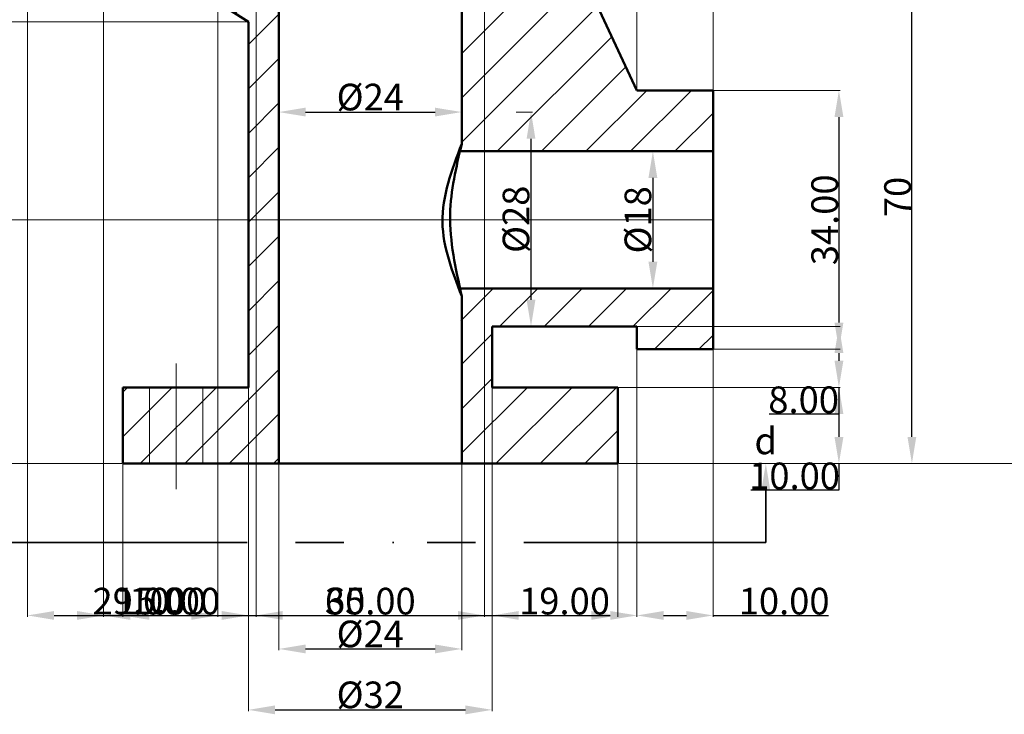
# Model space of a CAD drawing. Units: millimetres. Extents: x 75 to 489, y 21 to 350.
# Tile 3 of 5: x 142 to 271, y 176 to 268. Entities that reach past the tile are written whole.
import ezdxf

# ---------------------------------------------------------------- set-up
doc = ezdxf.new("R2010")
doc.units = ezdxf.units.MM
doc.header["$MEASUREMENT"] = 0
doc.linetypes.add('CENTER', pattern=[50.8, 31.75, -6.35, 6.35, -6.35])
doc.linetypes.add('PHANTOM', pattern=[63.5, 31.75, -6.35, 6.35, -6.35, 6.35, -6.35])
for name, color, linetype, lineweight in [('M-CNTR', 1, 'CENTER', 18), ('M-DIMS', 2, 'Continuous', 25), ('M-HATC', 8, 'Continuous', 18), ('M-OUTL', 7, 'Continuous', 50), ('M-SECT', 3, 'PHANTOM', 35), ('M-TEXT', 7, 'Continuous', 25), ('M-THRD', 3, 'Continuous', 18)]:
    doc.layers.add(name, color=color, linetype=linetype, lineweight=lineweight)
doc.styles.get("Standard").update_dxf_attribs({"font": 'arial.ttf'})
doc.dimstyles.get("Standard").update_dxf_attribs({"dimtxt": 3.5, "dimasz": 3.5, "dimexe": 0.18, "dimexo": 0.0625, "dimgap": 0.09, "dimtad": 1, "dimtoh": 1, "dimdec": 0, "dimzin": 0, "dimdsep": 46, "dimtxsty": 'Standard', "dimcen": 0.09, "dimclrd": 2, "dimclre": 251, "dimadec": 0, "dimazin": 0, "dimtfac": 1, "dimtdec": 0, "dimtofl": 0, "dimtmove": 0, "dimatfit": 3, "dimfxl": 1, "dimtolj": 1, "dimtzin": 0, "dimlwe": 5, "dimarcsym": 0})

# ---------------------------------------------------------------- blocks, each defined once
blk = doc.blocks.new('*D19')
at = {"layer": 'Defpoints', "color": 0, "transparency": 16777216}
for p in [(203.9, 223.35), (171.9, 219.35), (203.9, 177)]:
    blk.add_point(p, dxfattribs=at)
at = {"layer": 'M-DIMS', "color": 0, "lineweight": 5, "transparency": 16777216}
for p, q in [((203.9, 223.28), (203.9, 176.82)), ((171.9, 219.28), (171.9, 176.82))]:
    blk.add_line(p, q, dxfattribs=at)
at = {"layer": 'M-DIMS', "color": 0, "lineweight": -2, "transparency": 16777216}
blk.add_line((175.4, 177), (200.4, 177), dxfattribs=at)
at = {"layer": 'M-DIMS', "color": 0, "transparency": 16777216}
for points in [[(175.4, 177.58), (175.4, 176.42), (171.9, 177)], [(200.4, 177.58), (200.4, 176.42), (203.9, 177)]]:
    blk.add_solid(points, dxfattribs=at)
at = {"layer": 'M-DIMS', "color": 0, "transparency": 16777216, "insert": (187.9, 178.97), "char_height": 3.5, "attachment_point": 5}
blk.add_mtext('\\A1;%%C32', dxfattribs=at)
blk = doc.blocks.new('*D20')
at = {"layer": 'Defpoints', "color": 0, "transparency": 16777216}
for p in [(175.9, 216), (199.9, 216), (199.9, 185)]:
    blk.add_point(p, dxfattribs=at)
at = {"layer": 'M-DIMS', "color": 0, "lineweight": 5, "transparency": 16777216}
for p, q in [((175.9, 215.94), (175.9, 184.82)), ((199.9, 215.94), (199.9, 184.82))]:
    blk.add_line(p, q, dxfattribs=at)
at = {"layer": 'M-DIMS', "color": 0, "lineweight": -2, "transparency": 16777216}
blk.add_line((179.4, 185), (196.4, 185), dxfattribs=at)
at = {"layer": 'M-DIMS', "color": 0, "transparency": 16777216}
for points in [[(179.4, 185.58), (179.4, 184.42), (175.9, 185)], [(196.4, 185.58), (196.4, 184.42), (199.9, 185)]]:
    blk.add_solid(points, dxfattribs=at)
at = {"layer": 'M-DIMS', "color": 0, "transparency": 16777216, "insert": (187.9, 186.97), "char_height": 3.5, "attachment_point": 5}
blk.add_mtext('\\A1;%%C24', dxfattribs=at)
blk = doc.blocks.new('*D25')
at = {"layer": 'Defpoints', "color": 0, "transparency": 16777216}
for p in [(142.9, 299.35), (125.5, 241.35), (232.9, 241.35)]:
    blk.add_point(p, dxfattribs=at)
at = {"layer": 'M-DIMS', "color": 0, "lineweight": 5, "transparency": 16777216}
for p, q in [((142.84, 299.35), (125.32, 299.35)), ((232.84, 241.35), (125.32, 241.35))]:
    blk.add_line(p, q, dxfattribs=at)
at = {"layer": 'M-DIMS', "color": 0, "lineweight": -2, "transparency": 16777216}
blk.add_line((125.5, 295.85), (125.5, 244.85), dxfattribs=at)
at = {"layer": 'M-DIMS', "color": 0, "transparency": 16777216}
for points in [[(124.92, 295.85), (126.08, 295.85), (125.5, 299.35)], [(124.92, 244.85), (126.08, 244.85), (125.5, 241.35)]]:
    blk.add_solid(points, dxfattribs=at)
at = {"layer": 'M-DIMS', "color": 0, "transparency": 16777216, "insert": (123.62, 270.35), "char_height": 3.5, "attachment_point": 5, "rotation": 90}
blk.add_mtext('\\A1;58', dxfattribs=at)
blk = doc.blocks.new('*D26')
at = {"layer": 'Defpoints', "color": 0, "transparency": 16777216}
for p in [(117, 299.35), (142.9, 299.35), (155.4, 209.35)]:
    blk.add_point(p, dxfattribs=at)
at = {"layer": 'M-DIMS', "color": 0, "lineweight": 5, "transparency": 16777216}
for p, q in [((142.84, 299.35), (116.82, 299.35)), ((155.34, 209.35), (116.82, 209.35))]:
    blk.add_line(p, q, dxfattribs=at)
at = {"layer": 'M-DIMS', "color": 0, "lineweight": -2, "transparency": 16777216}
blk.add_line((117, 212.85), (117, 295.85), dxfattribs=at)
at = {"layer": 'M-DIMS', "color": 0, "transparency": 16777216}
for points in [[(116.42, 295.85), (117.58, 295.85), (117, 299.35)], [(116.42, 212.85), (117.58, 212.85), (117, 209.35)]]:
    blk.add_solid(points, dxfattribs=at)
at = {"layer": 'M-DIMS', "color": 0, "transparency": 16777216, "insert": (115.12, 254.35), "char_height": 3.5, "attachment_point": 5, "rotation": 90}
blk.add_mtext('\\A1;90', dxfattribs=at)
blk = doc.blocks.new('*D27')
at = {"layer": 'Defpoints', "color": 0, "transparency": 16777216}
for p in [(171.9, 267.35), (134, 209.35), (155.4, 209.35)]:
    blk.add_point(p, dxfattribs=at)
at = {"layer": 'M-DIMS', "color": 0, "lineweight": 5, "transparency": 16777216}
for p, q in [((171.84, 267.35), (133.82, 267.35)), ((155.34, 209.35), (133.82, 209.35))]:
    blk.add_line(p, q, dxfattribs=at)
at = {"layer": 'M-DIMS', "color": 0, "lineweight": -2, "transparency": 16777216}
blk.add_line((134, 263.85), (134, 212.85), dxfattribs=at)
at = {"layer": 'M-DIMS', "color": 0, "transparency": 16777216}
for points in [[(133.42, 263.85), (134.58, 263.85), (134, 267.35)], [(133.42, 212.85), (134.58, 212.85), (134, 209.35)]]:
    blk.add_solid(points, dxfattribs=at)
at = {"layer": 'M-DIMS', "color": 0, "transparency": 16777216, "insert": (132.12, 238.35), "char_height": 3.5, "attachment_point": 5, "rotation": 90}
blk.add_mtext('\\A1;58', dxfattribs=at)
blk = doc.blocks.new('*D28')
at = {"layer": 'Defpoints', "color": 0, "transparency": 16777216}
for p in [(175.9, 255.5), (199.9, 255.5), (199.9, 255.5)]:
    blk.add_point(p, dxfattribs=at)
at = {"layer": 'M-DIMS', "color": 0, "lineweight": 5, "transparency": 16777216}
for p, q in [((175.9, 255.56), (175.9, 255.68)), ((199.9, 255.56), (199.9, 255.68))]:
    blk.add_line(p, q, dxfattribs=at)
at = {"layer": 'M-DIMS', "color": 0, "lineweight": -2, "transparency": 16777216}
blk.add_line((179.4, 255.5), (196.4, 255.5), dxfattribs=at)
at = {"layer": 'M-DIMS', "color": 0, "transparency": 16777216}
for points in [[(179.4, 256.08), (179.4, 254.92), (175.9, 255.5)], [(196.4, 256.08), (196.4, 254.92), (199.9, 255.5)]]:
    blk.add_solid(points, dxfattribs=at)
at = {"layer": 'M-DIMS', "color": 0, "transparency": 16777216, "insert": (187.9, 257.47), "char_height": 3.5, "attachment_point": 5}
blk.add_mtext('\\A1;%%C24', dxfattribs=at)
blk = doc.blocks.new('*D29')
at = {"layer": 'Defpoints', "color": 0, "transparency": 16777216}
for p in [(228.5, 250.35), (225, 232.35), (228.5, 232.35)]:
    blk.add_point(p, dxfattribs=at)
at = {"layer": 'M-DIMS', "color": 0, "lineweight": 5, "transparency": 16777216}
for p, q in [((228.44, 250.35), (224.82, 250.35)), ((228.44, 232.35), (224.82, 232.35))]:
    blk.add_line(p, q, dxfattribs=at)
at = {"layer": 'M-DIMS', "color": 0, "lineweight": -2, "transparency": 16777216}
blk.add_line((225, 246.85), (225, 235.85), dxfattribs=at)
at = {"layer": 'M-DIMS', "color": 0, "transparency": 16777216}
for points in [[(224.42, 246.85), (225.58, 246.85), (225, 250.35)], [(224.42, 235.85), (225.58, 235.85), (225, 232.35)]]:
    blk.add_solid(points, dxfattribs=at)
at = {"layer": 'M-DIMS', "color": 0, "transparency": 16777216, "insert": (223.03, 241.35), "char_height": 3.5, "width": 5.2587, "attachment_point": 5, "rotation": 90}
blk.add_mtext('\\A1;%%C18', dxfattribs=at)
blk = doc.blocks.new('*D30')
at = {"layer": 'Defpoints', "color": 0, "transparency": 16777216}
for p in [(207, 255.5), (209, 255.5), (207, 227.35)]:
    blk.add_point(p, dxfattribs=at)
at = {"layer": 'M-DIMS', "color": 0, "lineweight": 5, "transparency": 16777216}
for p, q in [((207.06, 255.5), (209.18, 255.5)), ((207.06, 227.35), (209.18, 227.35))]:
    blk.add_line(p, q, dxfattribs=at)
at = {"layer": 'M-DIMS', "color": 0, "lineweight": -2, "transparency": 16777216}
blk.add_line((209, 230.85), (209, 252), dxfattribs=at)
at = {"layer": 'M-DIMS', "color": 0, "transparency": 16777216}
for points in [[(208.42, 252), (209.58, 252), (209, 255.5)], [(208.42, 230.85), (209.58, 230.85), (209, 227.35)]]:
    blk.add_solid(points, dxfattribs=at)
at = {"layer": 'M-DIMS', "color": 0, "transparency": 16777216, "insert": (207.03, 241.42), "char_height": 3.5, "attachment_point": 5, "rotation": 90}
blk.add_mtext('\\A1;%%C28', dxfattribs=at)
blk = doc.blocks.new('*D31')
at = {"layer": 'Defpoints', "color": 0, "transparency": 16777216}
for p in [(199.9, 279.35), (259, 279.35), (220.4, 209.35)]:
    blk.add_point(p, dxfattribs=at)
at = {"layer": 'M-DIMS', "color": 0, "lineweight": 5, "transparency": 16777216}
for p, q in [((199.97, 279.35), (259.18, 279.35)), ((220.47, 209.35), (259.18, 209.35))]:
    blk.add_line(p, q, dxfattribs=at)
at = {"layer": 'M-DIMS', "color": 0, "lineweight": -2, "transparency": 16777216}
blk.add_line((259, 212.85), (259, 275.85), dxfattribs=at)
at = {"layer": 'M-DIMS', "color": 0, "transparency": 16777216}
for points in [[(258.42, 275.85), (259.58, 275.85), (259, 279.35)], [(258.42, 212.85), (259.58, 212.85), (259, 209.35)]]:
    blk.add_solid(points, dxfattribs=at)
at = {"layer": 'M-DIMS', "color": 0, "transparency": 16777216, "insert": (257.12, 244.35), "char_height": 3.5, "attachment_point": 5, "rotation": 90}
blk.add_mtext('\\A1;70', dxfattribs=at)
blk = doc.blocks.new('*D35')
at = {"layer": 'Defpoints', "color": 0, "transparency": 16777216}
for p in [(220.88, 327.35), (259, 209.35), (279.5, 209.35)]:
    blk.add_point(p, dxfattribs=at)
at = {"layer": 'M-DIMS', "color": 0, "lineweight": 5, "transparency": 16777216}
for p, q in [((220.95, 327.35), (279.68, 327.35)), ((259.06, 209.35), (279.68, 209.35))]:
    blk.add_line(p, q, dxfattribs=at)
at = {"layer": 'M-DIMS', "color": 0, "lineweight": -2, "transparency": 16777216}
blk.add_line((279.5, 323.85), (279.5, 212.85), dxfattribs=at)
at = {"layer": 'M-DIMS', "color": 0, "transparency": 16777216}
for points in [[(278.92, 323.85), (280.08, 323.85), (279.5, 327.35)], [(278.92, 212.85), (280.08, 212.85), (279.5, 209.35)]]:
    blk.add_solid(points, dxfattribs=at)
at = {"layer": 'M-DIMS', "color": 0, "transparency": 16777216, "insert": (277.62, 268.35), "char_height": 3.5, "attachment_point": 5, "rotation": 90}
blk.add_mtext('\\A1;118', dxfattribs=at)
blk = doc.blocks.new('*D44')
at = {"layer": 'Defpoints', "color": 0, "transparency": 16777216}
for p in [(232.9, 345.6), (142.9, 319.35), (232.9, 258.35)]:
    blk.add_point(p, dxfattribs=at)
at = {"layer": 'M-DIMS', "color": 251, "lineweight": 5, "transparency": 16777216}
for p, q in [((142.9, 319.41), (142.9, 345.78)), ((232.9, 258.41), (232.9, 345.78))]:
    blk.add_line(p, q, dxfattribs=at)
at = {"layer": 'M-DIMS', "color": 2, "lineweight": -2, "transparency": 16777216}
blk.add_line((146.4, 345.6), (229.4, 345.6), dxfattribs=at)
at = {"layer": 'M-DIMS', "color": 2, "transparency": 16777216}
for points in [[(146.4, 346.18), (146.4, 345.02), (142.9, 345.6)], [(229.4, 346.18), (229.4, 345.02), (232.9, 345.6)]]:
    blk.add_solid(points, dxfattribs=at)
at = {"layer": 'M-DIMS', "color": 0, "transparency": 16777216, "insert": (187.9, 347.48), "char_height": 3.5, "attachment_point": 5}
blk.add_mtext('\\A1;90.00', dxfattribs=at)
blk = doc.blocks.new('*D47')
at = {"layer": 'Defpoints', "color": 0, "transparency": 16777216}
for p in [(155.4, 209.35), (220.4, 209.35), (220.4, 189.4)]:
    blk.add_point(p, dxfattribs=at)
at = {"layer": 'M-DIMS', "color": 251, "lineweight": 5, "transparency": 16777216}
for p, q in [((155.4, 209.28), (155.4, 189.22)), ((220.4, 209.28), (220.4, 189.22))]:
    blk.add_line(p, q, dxfattribs=at)
at = {"layer": 'M-DIMS', "color": 2, "lineweight": -2, "transparency": 16777216}
blk.add_line((158.9, 189.4), (216.9, 189.4), dxfattribs=at)
at = {"layer": 'M-DIMS', "color": 2, "transparency": 16777216}
for points in [[(158.9, 189.98), (158.9, 188.82), (155.4, 189.4)], [(216.9, 189.98), (216.9, 188.82), (220.4, 189.4)]]:
    blk.add_solid(points, dxfattribs=at)
at = {"layer": 'M-DIMS', "color": 0, "transparency": 16777216, "insert": (187.9, 191.28), "char_height": 3.5, "attachment_point": 5}
blk.add_mtext('\\A1;65.00', dxfattribs=at)
blk = doc.blocks.new('*D48')
at = {"layer": 'Defpoints', "color": 0, "transparency": 16777216}
for p in [(220.4, 219.35), (220.4, 209.35), (249.42, 209.35)]:
    blk.add_point(p, dxfattribs=at)
at = {"layer": 'M-DIMS', "color": 251, "lineweight": 5, "transparency": 16777216}
for p, q in [((220.47, 219.35), (249.6, 219.35)), ((220.47, 209.35), (249.6, 209.35))]:
    blk.add_line(p, q, dxfattribs=at)
at = {"layer": 'M-DIMS', "color": 2, "lineweight": -2, "transparency": 16777216}
for p, q in [((249.42, 215.85), (249.42, 212.85)), ((249.42, 209.35), (249.42, 205.85)), ((249.42, 205.85), (237.86, 205.85))]:
    blk.add_line(p, q, dxfattribs=at)
at = {"layer": 'M-DIMS', "color": 2, "transparency": 16777216}
for points in [[(248.84, 215.85), (250.01, 215.85), (249.42, 219.35)], [(248.84, 212.85), (250.01, 212.85), (249.42, 209.35)]]:
    blk.add_solid(points, dxfattribs=at)
at = {"layer": 'M-DIMS', "color": 0, "transparency": 16777216, "insert": (243.6, 207.72), "char_height": 3.5, "attachment_point": 5}
blk.add_mtext('\\A1;10.00', dxfattribs=at)
blk = doc.blocks.new('*D50')
at = {"layer": 'Defpoints', "color": 0, "transparency": 16777216}
for p in [(142.9, 279.35), (152.9, 279.35), (152.9, 189.4)]:
    blk.add_point(p, dxfattribs=at)
at = {"layer": 'M-DIMS', "color": 251, "lineweight": 5, "transparency": 16777216}
for p, q in [((142.9, 279.28), (142.9, 189.22)), ((152.9, 279.28), (152.9, 189.22))]:
    blk.add_line(p, q, dxfattribs=at)
at = {"layer": 'M-DIMS', "color": 2, "lineweight": -2, "transparency": 16777216}
for p, q in [((146.4, 189.4), (149.4, 189.4)), ((152.9, 189.4), (168.05, 189.4))]:
    blk.add_line(p, q, dxfattribs=at)
at = {"layer": 'M-DIMS', "color": 2, "transparency": 16777216}
for points in [[(146.4, 189.98), (146.4, 188.82), (142.9, 189.4)], [(149.4, 189.98), (149.4, 188.82), (152.9, 189.4)]]:
    blk.add_solid(points, dxfattribs=at)
at = {"layer": 'M-DIMS', "color": 0, "transparency": 16777216, "insert": (162.23, 191.28), "char_height": 3.5, "attachment_point": 5}
blk.add_mtext('\\A1;10.00', dxfattribs=at)
blk = doc.blocks.new('*D51')
at = {"layer": 'Defpoints', "color": 0, "transparency": 16777216}
for p in [(142.9, 279.35), (171.9, 267.35), (171.9, 189.4)]:
    blk.add_point(p, dxfattribs=at)
at = {"layer": 'M-DIMS', "color": 251, "lineweight": 5, "transparency": 16777216}
for p, q in [((142.9, 279.28), (142.9, 189.22)), ((171.9, 267.28), (171.9, 189.22))]:
    blk.add_line(p, q, dxfattribs=at)
at = {"layer": 'M-DIMS', "color": 2, "lineweight": -2, "transparency": 16777216}
blk.add_line((146.4, 189.4), (168.4, 189.4), dxfattribs=at)
at = {"layer": 'M-DIMS', "color": 2, "transparency": 16777216}
for points in [[(146.4, 189.98), (146.4, 188.82), (142.9, 189.4)], [(168.4, 189.98), (168.4, 188.82), (171.9, 189.4)]]:
    blk.add_solid(points, dxfattribs=at)
at = {"layer": 'M-DIMS', "color": 0, "transparency": 16777216, "insert": (157.4, 191.28), "char_height": 3.5, "attachment_point": 5}
blk.add_mtext('\\A1;29.00', dxfattribs=at)
blk = doc.blocks.new('*D52')
at = {"layer": 'Defpoints', "color": 0, "transparency": 16777216}
for p in [(222.9, 345.6), (207.9, 290.35), (222.9, 258.35)]:
    blk.add_point(p, dxfattribs=at)
at = {"layer": 'M-DIMS', "color": 251, "lineweight": 5, "transparency": 16777216}
for p, q in [((207.9, 290.41), (207.9, 345.78)), ((222.9, 258.41), (222.9, 345.78))]:
    blk.add_line(p, q, dxfattribs=at)
at = {"layer": 'M-DIMS', "color": 2, "lineweight": -2, "transparency": 16777216}
blk.add_line((211.4, 345.6), (219.4, 345.6), dxfattribs=at)
at = {"layer": 'M-DIMS', "color": 2, "transparency": 16777216}
for points in [[(211.4, 346.18), (211.4, 345.02), (207.9, 345.6)], [(219.4, 346.18), (219.4, 345.02), (222.9, 345.6)]]:
    blk.add_solid(points, dxfattribs=at)
at = {"layer": 'M-DIMS', "color": 0, "transparency": 16777216, "insert": (215.4, 347.48), "char_height": 3.5, "attachment_point": 5}
blk.add_mtext('\\A1;15.00', dxfattribs=at)
blk = doc.blocks.new('*D53')
at = {"layer": 'Defpoints', "color": 0, "transparency": 16777216}
for p in [(152.9, 315.35), (167.9, 315.35), (167.9, 189.4)]:
    blk.add_point(p, dxfattribs=at)
at = {"layer": 'M-DIMS', "color": 251, "lineweight": 5, "transparency": 16777216}
for p, q in [((152.9, 315.28), (152.9, 189.22)), ((167.9, 315.28), (167.9, 189.22))]:
    blk.add_line(p, q, dxfattribs=at)
at = {"layer": 'M-DIMS', "color": 2, "lineweight": -2, "transparency": 16777216}
blk.add_line((156.4, 189.4), (164.4, 189.4), dxfattribs=at)
at = {"layer": 'M-DIMS', "color": 2, "transparency": 16777216}
for points in [[(156.4, 189.98), (156.4, 188.82), (152.9, 189.4)], [(164.4, 189.98), (164.4, 188.82), (167.9, 189.4)]]:
    blk.add_solid(points, dxfattribs=at)
at = {"layer": 'M-DIMS', "color": 0, "transparency": 16777216, "insert": (160.4, 191.28), "char_height": 3.5, "attachment_point": 5}
blk.add_mtext('\\A1;15.00', dxfattribs=at)
blk = doc.blocks.new('*D54')
at = {"layer": 'Defpoints', "color": 0, "transparency": 16777216}
for p in [(232.9, 258.35), (232.9, 224.35), (249.42, 224.35)]:
    blk.add_point(p, dxfattribs=at)
at = {"layer": 'M-DIMS', "color": 251, "lineweight": 5, "transparency": 16777216}
for p, q in [((232.97, 258.35), (249.6, 258.35)), ((232.97, 224.35), (249.6, 224.35))]:
    blk.add_line(p, q, dxfattribs=at)
at = {"layer": 'M-DIMS', "color": 2, "lineweight": -2, "transparency": 16777216}
blk.add_line((249.42, 254.85), (249.42, 227.85), dxfattribs=at)
at = {"layer": 'M-DIMS', "color": 2, "transparency": 16777216}
for points in [[(248.84, 254.85), (250.01, 254.85), (249.42, 258.35)], [(248.84, 227.85), (250.01, 227.85), (249.42, 224.35)]]:
    blk.add_solid(points, dxfattribs=at)
at = {"layer": 'M-DIMS', "color": 0, "transparency": 16777216, "insert": (247.55, 241.35), "char_height": 3.5, "attachment_point": 5, "rotation": 90}
blk.add_mtext('\\A1;34.00', dxfattribs=at)
blk = doc.blocks.new('*D55')
at = {"layer": 'Defpoints', "color": 0, "transparency": 16777216}
for p in [(222.9, 224.35), (232.9, 224.35), (232.9, 189.4)]:
    blk.add_point(p, dxfattribs=at)
at = {"layer": 'M-DIMS', "color": 251, "lineweight": 5, "transparency": 16777216}
for p, q in [((222.9, 224.28), (222.9, 189.22)), ((232.9, 224.28), (232.9, 189.22))]:
    blk.add_line(p, q, dxfattribs=at)
at = {"layer": 'M-DIMS', "color": 2, "lineweight": -2, "transparency": 16777216}
for p, q in [((226.4, 189.4), (229.4, 189.4)), ((232.9, 189.4), (248.05, 189.4))]:
    blk.add_line(p, q, dxfattribs=at)
at = {"layer": 'M-DIMS', "color": 2, "transparency": 16777216}
for points in [[(226.4, 189.98), (226.4, 188.82), (222.9, 189.4)], [(229.4, 189.98), (229.4, 188.82), (232.9, 189.4)]]:
    blk.add_solid(points, dxfattribs=at)
at = {"layer": 'M-DIMS', "color": 0, "transparency": 16777216, "insert": (242.23, 191.28), "char_height": 3.5, "attachment_point": 5}
blk.add_mtext('\\A1;10.00', dxfattribs=at)
blk = doc.blocks.new('*D56')
at = {"layer": 'Defpoints', "color": 0, "transparency": 16777216}
for p in [(203.9, 227.35), (222.9, 227.35), (222.9, 189.4)]:
    blk.add_point(p, dxfattribs=at)
at = {"layer": 'M-DIMS', "color": 251, "lineweight": 5, "transparency": 16777216}
for p, q in [((203.9, 227.28), (203.9, 189.22)), ((222.9, 227.28), (222.9, 189.22))]:
    blk.add_line(p, q, dxfattribs=at)
at = {"layer": 'M-DIMS', "color": 2, "lineweight": -2, "transparency": 16777216}
blk.add_line((207.4, 189.4), (219.4, 189.4), dxfattribs=at)
at = {"layer": 'M-DIMS', "color": 2, "transparency": 16777216}
for points in [[(207.4, 189.98), (207.4, 188.82), (203.9, 189.4)], [(219.4, 189.98), (219.4, 188.82), (222.9, 189.4)]]:
    blk.add_solid(points, dxfattribs=at)
at = {"layer": 'M-DIMS', "color": 0, "transparency": 16777216, "insert": (213.4, 191.28), "char_height": 3.5, "attachment_point": 5}
blk.add_mtext('\\A1;19.00', dxfattribs=at)
blk = doc.blocks.new('*D57')
at = {"layer": 'Defpoints', "color": 0, "transparency": 16777216}
for p in [(172.9, 325.35), (202.9, 325.35), (202.9, 189.4)]:
    blk.add_point(p, dxfattribs=at)
at = {"layer": 'M-DIMS', "color": 251, "lineweight": 5, "transparency": 16777216}
for p, q in [((172.9, 325.28), (172.9, 189.22)), ((202.9, 325.28), (202.9, 189.22))]:
    blk.add_line(p, q, dxfattribs=at)
at = {"layer": 'M-DIMS', "color": 2, "lineweight": -2, "transparency": 16777216}
blk.add_line((176.4, 189.4), (199.4, 189.4), dxfattribs=at)
at = {"layer": 'M-DIMS', "color": 2, "transparency": 16777216}
for points in [[(176.4, 189.98), (176.4, 188.82), (172.9, 189.4)], [(199.4, 189.98), (199.4, 188.82), (202.9, 189.4)]]:
    blk.add_solid(points, dxfattribs=at)
at = {"layer": 'M-DIMS', "color": 0, "transparency": 16777216, "insert": (187.9, 191.28), "char_height": 3.5, "attachment_point": 5}
blk.add_mtext('\\A1;30.00', dxfattribs=at)
blk = doc.blocks.new('*D61')
at = {"layer": 'Defpoints', "color": 0, "transparency": 16777216}
for p in [(203.9, 227.35), (203.9, 219.35), (249.42, 219.35)]:
    blk.add_point(p, dxfattribs=at)
at = {"layer": 'M-DIMS', "color": 251, "lineweight": 5, "transparency": 16777216}
for p, q in [((203.97, 227.35), (249.6, 227.35)), ((203.97, 219.35), (249.6, 219.35))]:
    blk.add_line(p, q, dxfattribs=at)
at = {"layer": 'M-DIMS', "color": 2, "lineweight": -2, "transparency": 16777216}
for p, q in [((249.42, 223.85), (249.42, 222.85)), ((249.42, 219.35), (249.42, 215.85)), ((249.42, 215.85), (240.25, 215.85))]:
    blk.add_line(p, q, dxfattribs=at)
at = {"layer": 'M-DIMS', "color": 2, "transparency": 16777216}
for points in [[(248.84, 223.85), (250.01, 223.85), (249.42, 227.35)], [(248.84, 222.85), (250.01, 222.85), (249.42, 219.35)]]:
    blk.add_solid(points, dxfattribs=at)
at = {"layer": 'M-DIMS', "color": 0, "transparency": 16777216, "insert": (244.79, 217.72), "char_height": 3.5, "attachment_point": 5}
blk.add_mtext('\\A1;8.00', dxfattribs=at)

msp = doc.modelspace()

# ---------------------------------------------------------------- hatches: boundary and pattern name
at = {"layer": 'M-HATC'}
h = msp.add_hatch(dxfattribs=at)
h.set_pattern_fill('ANSI31', color=256, scale=33)
h.set_pattern_definition([(45, (-570, 152.5), (-2.916815, 2.916815), [])])
h.paths.add_polyline_path([(172.904, 325.347), (169.904, 325.347), (169.904, 327.347), (154.923, 327.347), (154.923, 319.347), (167.904, 319.347), (167.904, 315.347), (152.904, 315.347), (152.904, 319.347), (142.904, 319.347), (142.904, 310.347), (172.904, 310.347)])
h.paths.add_polyline_path([(220.885, 327.347), (205.904, 327.347), (205.904, 325.347), (202.904, 325.347), (202.904, 290.347), (201.904, 290.347), (201.904, 285.347), (197.904, 285.347), (197.904, 279.347), (199.904, 279.347), (199.904, 250.347), (232.904, 250.347), (232.904, 258.347), (222.904, 258.347), (207.904, 290.347), (207.904, 319.347), (220.885, 319.347)])
h.paths.add_polyline_path([(232.781, 232.347), (199.781, 232.347), (199.904, 209.347), (220.404, 209.347), (220.404, 219.347), (203.904, 219.347), (203.904, 227.347), (222.904, 227.347), (222.904, 224.347), (232.904, 224.347)])
h.paths.add_polyline_path([(175.904, 279.347), (177.904, 279.347), (177.904, 285.347), (172.904, 288.347), (142.904, 288.347), (142.904, 279.347), (152.904, 279.347), (171.904, 267.347), (171.904, 219.347), (155.404, 219.347), (155.404, 209.347), (175.904, 209.347)])

# ---------------------------------------------------------------- linework, layer by layer
at = {"layer": 'M-CNTR'}
msp.add_line((162.404, 206), (162.404, 222.5), dxfattribs=at)
at = {"layer": 'M-OUTL'}
for p, q in [((222.904, 258.347), (207.904, 290.347)), ((152.904, 279.347), (171.904, 267.347)), ((175.904, 279.347), (175.904, 209.347)), ((199.904, 251.347), (199.904, 279.347)), ((171.904, 267.347), (171.904, 219.347)), ((232.904, 258.347), (222.904, 258.347)), ((232.904, 224.347), (232.904, 258.347)), ((232.904, 250.347), (199.67, 250.347)), ((232.904, 232.347), (199.658, 232.347)), ((199.904, 209.347), (199.904, 231.347)), ((222.904, 227.347), (203.904, 227.347)), ((203.904, 227.347), (203.904, 219.347)), ((222.904, 224.347), (222.904, 227.347)), ((232.904, 224.347), (222.904, 224.347)), ((155.404, 219.347), (171.904, 219.347)), ((155.404, 209.347), (155.404, 219.347)), ((203.904, 219.347), (220.404, 219.347)), ((220.404, 219.347), (220.404, 209.347)), ((155.404, 209.347), (220.404, 209.347))]:
    msp.add_line(p, q, dxfattribs=at)
for points, knots in [([(199.904, 251.347), (198.613, 247.901), (196.108, 241.215), (198.665, 234.568), (199.904, 231.347)], [0, 0, 0, 0, 10.6337627, 20.6301077, 20.6301077, 20.6301077, 20.6301077]), ([(199.904, 251.347), (199.181, 248.264), (197.622, 241.614), (199.107, 234.931), (199.904, 231.347)], [0, 0, 0, 0, 9.3811748, 20.2292761, 20.2292761, 20.2292761, 20.2292761])]:
    msp.add_open_spline(points, degree=3, knots=knots, dxfattribs=at)
at = {"layer": 'M-SECT'}
for points in [[(140, 207.5), (140, 199), (191, 199)], [(239.823, 205.847), (239.823, 199), (191, 199)]]:
    msp.add_lwpolyline(points, dxfattribs=at)
msp.add_solid([(239.24, 205.847), (239.823, 209.347), (240.407, 205.847)], dxfattribs=at)
at = {"layer": 'M-THRD'}
for p, q in [((158.904, 209.347), (158.904, 219.347)), ((165.904, 209.347), (165.904, 219.347))]:
    msp.add_line(p, q, dxfattribs=at)

# ---------------------------------------------------------------- texts
at = {"layer": 'M-TEXT', "insert": (239.814, 212.323), "char_height": 3.5, "attachment_point": 5}
msp.add_mtext('\\A1;d', dxfattribs=at)

# ---------------------------------------------------------------- dimensions: what is measured, and where the dimension line sits
at = {"layer": 'M-DIMS'}
for base, p1, p2, picture, middle in [((232.904, 345.6), (142.904, 319.347), (232.904, 258.347), '*D44', (187.904, 347.477)), ((222.904, 345.6), (207.904, 290.347), (222.904, 258.347), '*D52', (215.404, 347.477)), ((202.904, 189.4), (172.904, 325.347), (202.904, 325.347), '*D57', (187.904, 191.278)), ((167.904, 189.4), (152.904, 315.347), (167.904, 315.347), '*D53', (160.404, 191.277)), ((152.904, 189.4), (142.904, 279.347), (152.904, 279.347), '*D50', (162.229, 191.277)), ((171.904, 189.4), (142.904, 279.347), (171.904, 267.347), '*D51', (157.404, 191.277)), ((222.904, 189.4), (203.904, 227.347), (222.904, 227.347), '*D56', (213.404, 191.277)), ((232.904, 189.4), (222.904, 224.347), (232.904, 224.347), '*D55', (242.229, 191.277)), ((220.404, 189.4), (155.404, 209.347), (220.404, 209.347), '*D47', (187.904, 191.277))]:
    dim = msp.add_linear_dim(base=base, p1=p1, p2=p2, dimstyle='Standard', override={"dimdec": 2, "dimlfac": 1, "dimrnd": 0, "dimzin": 0, "dimdsep": 46, "dimlunit": 2}, dxfattribs=at)
    dim.commit()
    dim.dimension.update_dxf_attribs({"geometry": picture, "text_midpoint": middle})
for base, p1, p2, override, picture, middle in [((279.5, 209.347), (220.885, 327.347), (259, 209.347), {"dimclrd": 0, "dimclre": 0, "dimclrt": 0}, '*D35', (277.623, 268.347)), ((117, 299.347), (155.404, 209.347), (142.904, 299.347), {"dimclrd": 0, "dimclre": 0, "dimclrt": 0}, '*D26', (115.123, 254.347)), ((125.5, 241.347), (142.904, 299.347), (232.904, 241.347), {"dimclrd": 0, "dimclre": 0, "dimclrt": 0}, '*D25', (123.623, 270.347)), ((259, 279.347), (220.404, 209.347), (199.904, 279.347), {"dimclrd": 0, "dimclre": 0, "dimclrt": 0}, '*D31', (257.123, 244.347)), ((134, 209.347), (171.904, 267.347), (155.404, 209.347), {"dimclrd": 0, "dimclre": 0, "dimclrt": 0}, '*D27', (132.123, 238.347)), ((249.423, 224.347), (232.904, 258.347), (232.904, 224.347), {"dimdec": 2, "dimlfac": 1, "dimrnd": 0, "dimzin": 0, "dimdsep": 46, "dimlunit": 2}, '*D54', (247.545, 241.347)), ((249.423, 219.347), (203.904, 227.347), (203.904, 219.347), {"dimdec": 2, "dimlfac": 1, "dimrnd": 0, "dimzin": 0, "dimdsep": 46, "dimlunit": 2}, '*D61', (244.791, 217.724)), ((249.423, 209.347), (220.404, 219.347), (220.404, 209.347), {"dimdec": 2, "dimlfac": 1, "dimrnd": 0, "dimzin": 0, "dimdsep": 46, "dimlunit": 2}, '*D48', (243.599, 207.724))]:
    dim = msp.add_linear_dim(base=base, p1=p1, p2=p2, angle=90, dimstyle='Standard', override=override, dxfattribs=at)
    dim.commit()
    dim.dimension.update_dxf_attribs({"geometry": picture, "text_midpoint": middle})
for base, p1, p2, picture, middle in [((199.904, 255.5), (175.904, 255.5), (199.904, 255.5), '*D28', (187.904, 257.475)), ((203.904, 177), (171.904, 219.347), (203.904, 223.347), '*D19', (187.904, 178.975)), ((199.904, 185), (175.904, 216), (199.904, 216), '*D20', (187.904, 186.975))]:
    dim = msp.add_linear_dim(base=base, p1=p1, p2=p2, text='%%C<>', dimstyle='Standard', override={"dimclrd": 0, "dimclre": 0, "dimclrt": 0}, dxfattribs=at)
    dim.commit()
    dim.dimension.update_dxf_attribs({"geometry": picture, "text_midpoint": middle})
for base, p1, p2, picture, middle in [((209, 255.5), (207, 227.347), (207, 255.5), '*D30', (207.025, 241.424)), ((225, 232.347), (228.5, 250.347), (228.5, 232.347), '*D29', (223.025, 241.347))]:
    dim = msp.add_linear_dim(base=base, p1=p1, p2=p2, angle=90, text='%%C<>', dimstyle='Standard', override={"dimclrd": 0, "dimclre": 0, "dimclrt": 0}, dxfattribs=at)
    dim.commit()
    dim.dimension.update_dxf_attribs({"geometry": picture, "text_midpoint": middle})

doc.saveas('drawing.dxf')
